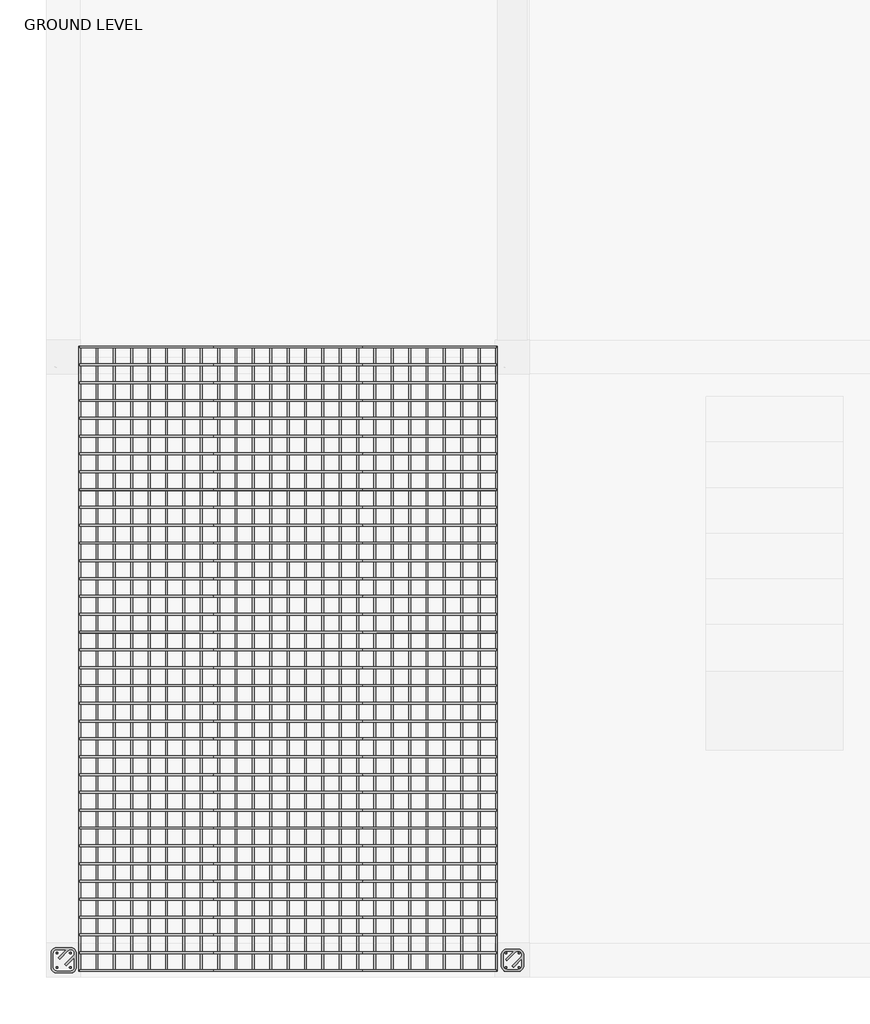
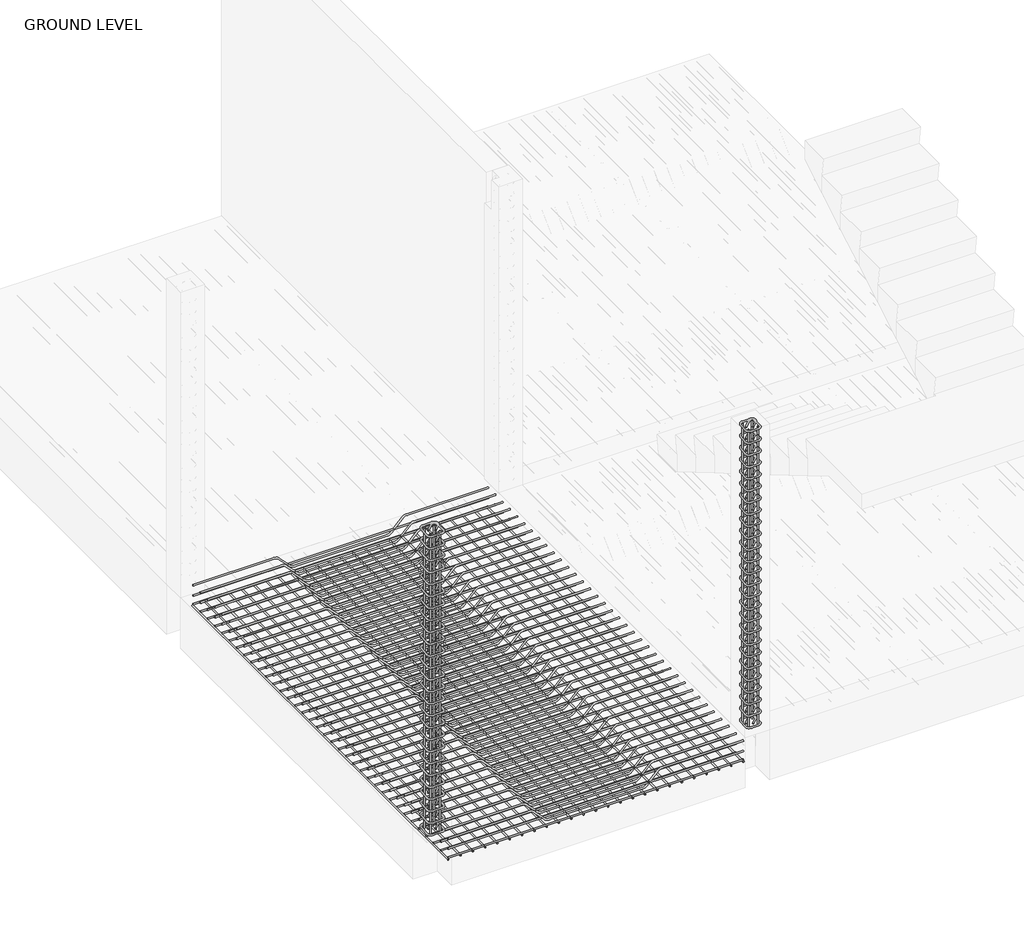
# One storey, part 2 of 8: 10 reinforcing bars.
"""IFC4 building model written with IfcOpenShell, lengths in millimetres."""

from ifc_helpers import new_model, si_unit, point, frame, origin, place, context, project, spatial, polyline, circle_curve, trimmed, segment, composite_curve, source, transform, mapped, element, save
from ifc_brep_helpers import swept_disk

model = new_model("IFC4")

# Units and contexts
model_context = context("Model", 3, world=origin())
ifc_project = project(units=[si_unit("LENGTHUNIT", "METRE", prefix="MILLI")], contexts=[model_context])

# Site, building, storey
site = spatial("IfcSite", under=ifc_project)
building = spatial("IfcBuilding", under=site)
storey = spatial("IfcBuildingStorey", under=building, Name="GROUND LEVEL", Elevation=0.0)

# Reinforcing bars
placement = place(None, origin())
reinforcing_bar_shape = source(origin(), model_context, "Body", "SolidModel", [
    swept_disk(composite_curve([segment(polyline([(-14816.7556793, -164.7525279, -60.0), (-14046.7544785, -164.7525279, -60.0)]), True, "CONTINUOUS"), segment(trimmed(circle_curve(frame((-14046.7544785, -164.7525279, -106.35), z_axis=(0.0, 1.0, 0.0), x_axis=(0.0, 0.0, 46.349999999999994)), 46.35), [point((-14046.7544785, -164.7525279, -60.0))], [point((-14013.9800792, -164.7525279, -73.5756007))], True, "CARTESIAN"), True, "CONTINUOUS"), segment(polyline([(-14013.9800792, -164.7525279, -73.5756007), (-13899.7099243, -164.7525279, -187.8457555)]), True, "CONTINUOUS"), segment(trimmed(circle_curve(frame((-13866.935525, -164.7525279, -155.0713562), z_axis=(0.0, -1.0, 0.0), x_axis=(-32.77439929999855, 0.0, -32.7743993)), 46.35), [point((-13899.7099243, -164.7525279, -187.8457555))], [point((-13866.935525, -164.7525279, -201.4213562))], True, "CARTESIAN"), True, "CONTINUOUS"), segment(polyline([(-13866.935525, -164.7525279, -201.4213562), (-12983.3758347, -164.7525279, -201.4213562)]), True, "CONTINUOUS"), segment(trimmed(circle_curve(frame((-12983.3758347, -164.7525279, -155.0713562), z_axis=(0.0, -1.0, 0.0), x_axis=(0.0, 0.0, -46.349999999999994)), 46.35), [point((-12983.3758347, -164.7525279, -201.4213562))], [point((-12950.6014354, -164.7525279, -187.8457555))], True, "CARTESIAN"), True, "CONTINUOUS"), segment(polyline([(-12950.6014354, -164.7525279, -187.8457555), (-12836.3312806, -164.7525279, -73.5756007)]), True, "CONTINUOUS"), segment(trimmed(circle_curve(frame((-12803.5568813, -164.7525279, -106.35), z_axis=(0.0, 1.0, 0.0), x_axis=(-32.77439929999855, 0.0, 32.7743993)), 46.35), [point((-12836.3312806, -164.7525279, -73.5756007))], [point((-12803.5568813, -164.7525279, -60.0))], True, "CARTESIAN"), True, "CONTINUOUS"), segment(polyline([(-12803.5568813, -164.7525279, -60.0), (-12033.5556805, -164.7525279, -60.0)]), True, "CONTINUOUS")], self_intersect=False), 6.35),
])
element("IfcReinforcingBar", 1, at=placement, inside=storey, context=model_context, shape_type="MappedRepresentation", body=[
    mapped(reinforcing_bar_shape, transform((0.0, 0.0, 0.0), x_axis=(1.0, 0.0, 0.0), y_axis=(0.0, 1.0, 0.0), z_axis=(0.0, 0.0, 1.0))),
    mapped(reinforcing_bar_shape, transform((0.0, -118.9455945, 0.0), x_axis=(1.0, 0.0, 0.0), y_axis=(0.0, 1.0, 0.0), z_axis=(0.0, 0.0, 1.0))),
    mapped(reinforcing_bar_shape, transform((0.0, -237.891189, 0.0), x_axis=(1.0, 0.0, 0.0), y_axis=(0.0, 1.0, 0.0), z_axis=(0.0, 0.0, 1.0))),
    mapped(reinforcing_bar_shape, transform((0.0, -356.8367835, 0.0), x_axis=(1.0, 0.0, 0.0), y_axis=(0.0, 1.0, 0.0), z_axis=(0.0, 0.0, 1.0))),
    mapped(reinforcing_bar_shape, transform((0.0, -475.7823779, 0.0), x_axis=(1.0, 0.0, 0.0), y_axis=(0.0, 1.0, 0.0), z_axis=(0.0, 0.0, 1.0))),
    mapped(reinforcing_bar_shape, transform((0.0, -594.7279724, 0.0), x_axis=(1.0, 0.0, 0.0), y_axis=(0.0, 1.0, 0.0), z_axis=(0.0, 0.0, 1.0))),
    mapped(reinforcing_bar_shape, transform((0.0, -713.6735669, 0.0), x_axis=(1.0, 0.0, 0.0), y_axis=(0.0, 1.0, 0.0), z_axis=(0.0, 0.0, 1.0))),
    mapped(reinforcing_bar_shape, transform((0.0, -832.6191614, 0.0), x_axis=(1.0, 0.0, 0.0), y_axis=(0.0, 1.0, 0.0), z_axis=(0.0, 0.0, 1.0))),
    mapped(reinforcing_bar_shape, transform((0.0, -951.5647559, 0.0), x_axis=(1.0, 0.0, 0.0), y_axis=(0.0, 1.0, 0.0), z_axis=(0.0, 0.0, 1.0))),
    mapped(reinforcing_bar_shape, transform((0.0, -1070.5103504, 0.0), x_axis=(1.0, 0.0, 0.0), y_axis=(0.0, 1.0, 0.0), z_axis=(0.0, 0.0, 1.0))),
    mapped(reinforcing_bar_shape, transform((0.0, -1189.4559449, 0.0), x_axis=(1.0, 0.0, 0.0), y_axis=(0.0, 1.0, 0.0), z_axis=(0.0, 0.0, 1.0))),
    mapped(reinforcing_bar_shape, transform((0.0, -1308.4015394, 0.0), x_axis=(1.0, 0.0, 0.0), y_axis=(0.0, 1.0, 0.0), z_axis=(0.0, 0.0, 1.0))),
    mapped(reinforcing_bar_shape, transform((0.0, -1427.3471338, 0.0), x_axis=(1.0, 0.0, 0.0), y_axis=(0.0, 1.0, 0.0), z_axis=(0.0, 0.0, 1.0))),
    mapped(reinforcing_bar_shape, transform((0.0, -1546.2927283, 0.0), x_axis=(1.0, 0.0, 0.0), y_axis=(0.0, 1.0, 0.0), z_axis=(0.0, 0.0, 1.0))),
    mapped(reinforcing_bar_shape, transform((0.0, -1665.2383228, 0.0), x_axis=(1.0, 0.0, 0.0), y_axis=(0.0, 1.0, 0.0), z_axis=(0.0, 0.0, 1.0))),
    mapped(reinforcing_bar_shape, transform((0.0, -1784.1839173, 0.0), x_axis=(1.0, 0.0, 0.0), y_axis=(0.0, 1.0, 0.0), z_axis=(0.0, 0.0, 1.0))),
    mapped(reinforcing_bar_shape, transform((0.0, -1903.1295118, 0.0), x_axis=(1.0, 0.0, 0.0), y_axis=(0.0, 1.0, 0.0), z_axis=(0.0, 0.0, 1.0))),
    mapped(reinforcing_bar_shape, transform((0.0, -2022.0751063, 0.0), x_axis=(1.0, 0.0, 0.0), y_axis=(0.0, 1.0, 0.0), z_axis=(0.0, 0.0, 1.0))),
    mapped(reinforcing_bar_shape, transform((0.0, -2141.0207008, 0.0), x_axis=(1.0, 0.0, 0.0), y_axis=(0.0, 1.0, 0.0), z_axis=(0.0, 0.0, 1.0))),
    mapped(reinforcing_bar_shape, transform((0.0, -2259.9662953, 0.0), x_axis=(1.0, 0.0, 0.0), y_axis=(0.0, 1.0, 0.0), z_axis=(0.0, 0.0, 1.0))),
    mapped(reinforcing_bar_shape, transform((0.0, -2378.9118897, 0.0), x_axis=(1.0, 0.0, 0.0), y_axis=(0.0, 1.0, 0.0), z_axis=(0.0, 0.0, 1.0))),
    mapped(reinforcing_bar_shape, transform((0.0, -2497.8574842, 0.0), x_axis=(1.0, 0.0, 0.0), y_axis=(0.0, 1.0, 0.0), z_axis=(0.0, 0.0, 1.0))),
    mapped(reinforcing_bar_shape, transform((0.0, -2616.8030787, 0.0), x_axis=(1.0, 0.0, 0.0), y_axis=(0.0, 1.0, 0.0), z_axis=(0.0, 0.0, 1.0))),
    mapped(reinforcing_bar_shape, transform((0.0, -2735.7486732, 0.0), x_axis=(1.0, 0.0, 0.0), y_axis=(0.0, 1.0, 0.0), z_axis=(0.0, 0.0, 1.0))),
    mapped(reinforcing_bar_shape, transform((0.0, -2854.6942677, 0.0), x_axis=(1.0, 0.0, 0.0), y_axis=(0.0, 1.0, 0.0), z_axis=(0.0, 0.0, 1.0))),
    mapped(reinforcing_bar_shape, transform((0.0, -2973.6398622, 0.0), x_axis=(1.0, 0.0, 0.0), y_axis=(0.0, 1.0, 0.0), z_axis=(0.0, 0.0, 1.0))),
    mapped(reinforcing_bar_shape, transform((0.0, -3092.5854567, 0.0), x_axis=(1.0, 0.0, 0.0), y_axis=(0.0, 1.0, 0.0), z_axis=(0.0, 0.0, 1.0))),
    mapped(reinforcing_bar_shape, transform((0.0, -3211.5310511, 0.0), x_axis=(1.0, 0.0, 0.0), y_axis=(0.0, 1.0, 0.0), z_axis=(0.0, 0.0, 1.0))),
    mapped(reinforcing_bar_shape, transform((0.0, -3330.4766456, 0.0), x_axis=(1.0, 0.0, 0.0), y_axis=(0.0, 1.0, 0.0), z_axis=(0.0, 0.0, 1.0))),
    mapped(reinforcing_bar_shape, transform((0.0, -3449.4222401, 0.0), x_axis=(1.0, 0.0, 0.0), y_axis=(0.0, 1.0, 0.0), z_axis=(0.0, 0.0, 1.0))),
    mapped(reinforcing_bar_shape, transform((0.0, -3568.3678346, 0.0), x_axis=(1.0, 0.0, 0.0), y_axis=(0.0, 1.0, 0.0), z_axis=(0.0, 0.0, 1.0))),
    mapped(reinforcing_bar_shape, transform((0.0, -3687.3134291, 0.0), x_axis=(1.0, 0.0, 0.0), y_axis=(0.0, 1.0, 0.0), z_axis=(0.0, 0.0, 1.0))),
    mapped(reinforcing_bar_shape, transform((0.0, -3806.2590236, 0.0), x_axis=(1.0, 0.0, 0.0), y_axis=(0.0, 1.0, 0.0), z_axis=(0.0, 0.0, 1.0))),
    mapped(reinforcing_bar_shape, transform((0.0, -3925.2046181, 0.0), x_axis=(1.0, 0.0, 0.0), y_axis=(0.0, 1.0, 0.0), z_axis=(0.0, 0.0, 1.0))),
    mapped(reinforcing_bar_shape, transform((0.0, -4044.1502126, 0.0), x_axis=(1.0, 0.0, 0.0), y_axis=(0.0, 1.0, 0.0), z_axis=(0.0, 0.0, 1.0))),
    mapped(reinforcing_bar_shape, transform((0.0, -4163.095807, 0.0), x_axis=(1.0, 0.0, 0.0), y_axis=(0.0, 1.0, 0.0), z_axis=(0.0, 0.0, 1.0))),
])
reinforcing_bar_2_shape = source(origin(), model_context, "Body", "SolidModel", [
    swept_disk(composite_curve([segment(polyline([(-12033.5556805, -164.7525279, -249.9712592), (-14816.7556793, -164.7525279, -249.9712592)]), True, "CONTINUOUS")], self_intersect=False), 6.35),
])
element("IfcReinforcingBar", 2, at=placement, inside=storey, context=model_context, shape_type="MappedRepresentation", body=[
    mapped(reinforcing_bar_2_shape, transform((0.0, 0.0, 0.0), x_axis=(1.0, 0.0, 0.0), y_axis=(0.0, 1.0, 0.0), z_axis=(0.0, 0.0, 1.0))),
    mapped(reinforcing_bar_2_shape, transform((0.0, -118.9455945, 0.0), x_axis=(1.0, 0.0, 0.0), y_axis=(0.0, 1.0, 0.0), z_axis=(0.0, 0.0, 1.0))),
    mapped(reinforcing_bar_2_shape, transform((0.0, -237.891189, 0.0), x_axis=(1.0, 0.0, 0.0), y_axis=(0.0, 1.0, 0.0), z_axis=(0.0, 0.0, 1.0))),
    mapped(reinforcing_bar_2_shape, transform((0.0, -356.8367835, 0.0), x_axis=(1.0, 0.0, 0.0), y_axis=(0.0, 1.0, 0.0), z_axis=(0.0, 0.0, 1.0))),
    mapped(reinforcing_bar_2_shape, transform((0.0, -475.7823779, 0.0), x_axis=(1.0, 0.0, 0.0), y_axis=(0.0, 1.0, 0.0), z_axis=(0.0, 0.0, 1.0))),
    mapped(reinforcing_bar_2_shape, transform((0.0, -594.7279724, 0.0), x_axis=(1.0, 0.0, 0.0), y_axis=(0.0, 1.0, 0.0), z_axis=(0.0, 0.0, 1.0))),
    mapped(reinforcing_bar_2_shape, transform((0.0, -713.6735669, 0.0), x_axis=(1.0, 0.0, 0.0), y_axis=(0.0, 1.0, 0.0), z_axis=(0.0, 0.0, 1.0))),
    mapped(reinforcing_bar_2_shape, transform((0.0, -832.6191614, 0.0), x_axis=(1.0, 0.0, 0.0), y_axis=(0.0, 1.0, 0.0), z_axis=(0.0, 0.0, 1.0))),
    mapped(reinforcing_bar_2_shape, transform((0.0, -951.5647559, 0.0), x_axis=(1.0, 0.0, 0.0), y_axis=(0.0, 1.0, 0.0), z_axis=(0.0, 0.0, 1.0))),
    mapped(reinforcing_bar_2_shape, transform((0.0, -1070.5103504, 0.0), x_axis=(1.0, 0.0, 0.0), y_axis=(0.0, 1.0, 0.0), z_axis=(0.0, 0.0, 1.0))),
    mapped(reinforcing_bar_2_shape, transform((0.0, -1189.4559449, 0.0), x_axis=(1.0, 0.0, 0.0), y_axis=(0.0, 1.0, 0.0), z_axis=(0.0, 0.0, 1.0))),
    mapped(reinforcing_bar_2_shape, transform((0.0, -1308.4015394, 0.0), x_axis=(1.0, 0.0, 0.0), y_axis=(0.0, 1.0, 0.0), z_axis=(0.0, 0.0, 1.0))),
    mapped(reinforcing_bar_2_shape, transform((0.0, -1427.3471338, 0.0), x_axis=(1.0, 0.0, 0.0), y_axis=(0.0, 1.0, 0.0), z_axis=(0.0, 0.0, 1.0))),
    mapped(reinforcing_bar_2_shape, transform((0.0, -1546.2927283, 0.0), x_axis=(1.0, 0.0, 0.0), y_axis=(0.0, 1.0, 0.0), z_axis=(0.0, 0.0, 1.0))),
    mapped(reinforcing_bar_2_shape, transform((0.0, -1665.2383228, 0.0), x_axis=(1.0, 0.0, 0.0), y_axis=(0.0, 1.0, 0.0), z_axis=(0.0, 0.0, 1.0))),
    mapped(reinforcing_bar_2_shape, transform((0.0, -1784.1839173, 0.0), x_axis=(1.0, 0.0, 0.0), y_axis=(0.0, 1.0, 0.0), z_axis=(0.0, 0.0, 1.0))),
    mapped(reinforcing_bar_2_shape, transform((0.0, -1903.1295118, 0.0), x_axis=(1.0, 0.0, 0.0), y_axis=(0.0, 1.0, 0.0), z_axis=(0.0, 0.0, 1.0))),
    mapped(reinforcing_bar_2_shape, transform((0.0, -2022.0751063, 0.0), x_axis=(1.0, 0.0, 0.0), y_axis=(0.0, 1.0, 0.0), z_axis=(0.0, 0.0, 1.0))),
    mapped(reinforcing_bar_2_shape, transform((0.0, -2141.0207008, 0.0), x_axis=(1.0, 0.0, 0.0), y_axis=(0.0, 1.0, 0.0), z_axis=(0.0, 0.0, 1.0))),
    mapped(reinforcing_bar_2_shape, transform((0.0, -2259.9662953, 0.0), x_axis=(1.0, 0.0, 0.0), y_axis=(0.0, 1.0, 0.0), z_axis=(0.0, 0.0, 1.0))),
    mapped(reinforcing_bar_2_shape, transform((0.0, -2378.9118897, 0.0), x_axis=(1.0, 0.0, 0.0), y_axis=(0.0, 1.0, 0.0), z_axis=(0.0, 0.0, 1.0))),
    mapped(reinforcing_bar_2_shape, transform((0.0, -2497.8574842, 0.0), x_axis=(1.0, 0.0, 0.0), y_axis=(0.0, 1.0, 0.0), z_axis=(0.0, 0.0, 1.0))),
    mapped(reinforcing_bar_2_shape, transform((0.0, -2616.8030787, 0.0), x_axis=(1.0, 0.0, 0.0), y_axis=(0.0, 1.0, 0.0), z_axis=(0.0, 0.0, 1.0))),
    mapped(reinforcing_bar_2_shape, transform((0.0, -2735.7486732, 0.0), x_axis=(1.0, 0.0, 0.0), y_axis=(0.0, 1.0, 0.0), z_axis=(0.0, 0.0, 1.0))),
    mapped(reinforcing_bar_2_shape, transform((0.0, -2854.6942677, 0.0), x_axis=(1.0, 0.0, 0.0), y_axis=(0.0, 1.0, 0.0), z_axis=(0.0, 0.0, 1.0))),
    mapped(reinforcing_bar_2_shape, transform((0.0, -2973.6398622, 0.0), x_axis=(1.0, 0.0, 0.0), y_axis=(0.0, 1.0, 0.0), z_axis=(0.0, 0.0, 1.0))),
    mapped(reinforcing_bar_2_shape, transform((0.0, -3092.5854567, 0.0), x_axis=(1.0, 0.0, 0.0), y_axis=(0.0, 1.0, 0.0), z_axis=(0.0, 0.0, 1.0))),
    mapped(reinforcing_bar_2_shape, transform((0.0, -3211.5310511, 0.0), x_axis=(1.0, 0.0, 0.0), y_axis=(0.0, 1.0, 0.0), z_axis=(0.0, 0.0, 1.0))),
    mapped(reinforcing_bar_2_shape, transform((0.0, -3330.4766456, 0.0), x_axis=(1.0, 0.0, 0.0), y_axis=(0.0, 1.0, 0.0), z_axis=(0.0, 0.0, 1.0))),
    mapped(reinforcing_bar_2_shape, transform((0.0, -3449.4222401, 0.0), x_axis=(1.0, 0.0, 0.0), y_axis=(0.0, 1.0, 0.0), z_axis=(0.0, 0.0, 1.0))),
    mapped(reinforcing_bar_2_shape, transform((0.0, -3568.3678346, 0.0), x_axis=(1.0, 0.0, 0.0), y_axis=(0.0, 1.0, 0.0), z_axis=(0.0, 0.0, 1.0))),
    mapped(reinforcing_bar_2_shape, transform((0.0, -3687.3134291, 0.0), x_axis=(1.0, 0.0, 0.0), y_axis=(0.0, 1.0, 0.0), z_axis=(0.0, 0.0, 1.0))),
    mapped(reinforcing_bar_2_shape, transform((0.0, -3806.2590236, 0.0), x_axis=(1.0, 0.0, 0.0), y_axis=(0.0, 1.0, 0.0), z_axis=(0.0, 0.0, 1.0))),
    mapped(reinforcing_bar_2_shape, transform((0.0, -3925.2046181, 0.0), x_axis=(1.0, 0.0, 0.0), y_axis=(0.0, 1.0, 0.0), z_axis=(0.0, 0.0, 1.0))),
    mapped(reinforcing_bar_2_shape, transform((0.0, -4044.1502126, 0.0), x_axis=(1.0, 0.0, 0.0), y_axis=(0.0, 1.0, 0.0), z_axis=(0.0, 0.0, 1.0))),
    mapped(reinforcing_bar_2_shape, transform((0.0, -4163.095807, 0.0), x_axis=(1.0, 0.0, 0.0), y_axis=(0.0, 1.0, 0.0), z_axis=(0.0, 0.0, 1.0))),
])
reinforcing_bar_3_shape = source(origin(), model_context, "Body", "SolidModel", [
    swept_disk(composite_curve([segment(polyline([(-14816.7556793, -164.7525279, -161.5623157), (-12033.5556805, -164.7525279, -161.5623157)]), True, "CONTINUOUS")], self_intersect=False), 6.35),
])
element("IfcReinforcingBar", 3, at=placement, inside=storey, context=model_context, shape_type="MappedRepresentation", body=[
    mapped(reinforcing_bar_3_shape, transform((0.0, 0.0, 0.0), x_axis=(1.0, 0.0, 0.0), y_axis=(0.0, 1.0, 0.0), z_axis=(0.0, 0.0, 1.0))),
    mapped(reinforcing_bar_3_shape, transform((0.0, -118.9455945, 0.0), x_axis=(1.0, 0.0, 0.0), y_axis=(0.0, 1.0, 0.0), z_axis=(0.0, 0.0, 1.0))),
    mapped(reinforcing_bar_3_shape, transform((0.0, -237.891189, 0.0), x_axis=(1.0, 0.0, 0.0), y_axis=(0.0, 1.0, 0.0), z_axis=(0.0, 0.0, 1.0))),
    mapped(reinforcing_bar_3_shape, transform((0.0, -356.8367835, 0.0), x_axis=(1.0, 0.0, 0.0), y_axis=(0.0, 1.0, 0.0), z_axis=(0.0, 0.0, 1.0))),
    mapped(reinforcing_bar_3_shape, transform((0.0, -475.7823779, 0.0), x_axis=(1.0, 0.0, 0.0), y_axis=(0.0, 1.0, 0.0), z_axis=(0.0, 0.0, 1.0))),
    mapped(reinforcing_bar_3_shape, transform((0.0, -594.7279724, 0.0), x_axis=(1.0, 0.0, 0.0), y_axis=(0.0, 1.0, 0.0), z_axis=(0.0, 0.0, 1.0))),
    mapped(reinforcing_bar_3_shape, transform((0.0, -713.6735669, 0.0), x_axis=(1.0, 0.0, 0.0), y_axis=(0.0, 1.0, 0.0), z_axis=(0.0, 0.0, 1.0))),
    mapped(reinforcing_bar_3_shape, transform((0.0, -832.6191614, 0.0), x_axis=(1.0, 0.0, 0.0), y_axis=(0.0, 1.0, 0.0), z_axis=(0.0, 0.0, 1.0))),
    mapped(reinforcing_bar_3_shape, transform((0.0, -951.5647559, 0.0), x_axis=(1.0, 0.0, 0.0), y_axis=(0.0, 1.0, 0.0), z_axis=(0.0, 0.0, 1.0))),
    mapped(reinforcing_bar_3_shape, transform((0.0, -1070.5103504, 0.0), x_axis=(1.0, 0.0, 0.0), y_axis=(0.0, 1.0, 0.0), z_axis=(0.0, 0.0, 1.0))),
    mapped(reinforcing_bar_3_shape, transform((0.0, -1189.4559449, 0.0), x_axis=(1.0, 0.0, 0.0), y_axis=(0.0, 1.0, 0.0), z_axis=(0.0, 0.0, 1.0))),
    mapped(reinforcing_bar_3_shape, transform((0.0, -1308.4015394, 0.0), x_axis=(1.0, 0.0, 0.0), y_axis=(0.0, 1.0, 0.0), z_axis=(0.0, 0.0, 1.0))),
    mapped(reinforcing_bar_3_shape, transform((0.0, -1427.3471338, 0.0), x_axis=(1.0, 0.0, 0.0), y_axis=(0.0, 1.0, 0.0), z_axis=(0.0, 0.0, 1.0))),
    mapped(reinforcing_bar_3_shape, transform((0.0, -1546.2927283, 0.0), x_axis=(1.0, 0.0, 0.0), y_axis=(0.0, 1.0, 0.0), z_axis=(0.0, 0.0, 1.0))),
    mapped(reinforcing_bar_3_shape, transform((0.0, -1665.2383228, 0.0), x_axis=(1.0, 0.0, 0.0), y_axis=(0.0, 1.0, 0.0), z_axis=(0.0, 0.0, 1.0))),
    mapped(reinforcing_bar_3_shape, transform((0.0, -1784.1839173, 0.0), x_axis=(1.0, 0.0, 0.0), y_axis=(0.0, 1.0, 0.0), z_axis=(0.0, 0.0, 1.0))),
    mapped(reinforcing_bar_3_shape, transform((0.0, -1903.1295118, 0.0), x_axis=(1.0, 0.0, 0.0), y_axis=(0.0, 1.0, 0.0), z_axis=(0.0, 0.0, 1.0))),
    mapped(reinforcing_bar_3_shape, transform((0.0, -2022.0751063, 0.0), x_axis=(1.0, 0.0, 0.0), y_axis=(0.0, 1.0, 0.0), z_axis=(0.0, 0.0, 1.0))),
    mapped(reinforcing_bar_3_shape, transform((0.0, -2141.0207008, 0.0), x_axis=(1.0, 0.0, 0.0), y_axis=(0.0, 1.0, 0.0), z_axis=(0.0, 0.0, 1.0))),
    mapped(reinforcing_bar_3_shape, transform((0.0, -2259.9662953, 0.0), x_axis=(1.0, 0.0, 0.0), y_axis=(0.0, 1.0, 0.0), z_axis=(0.0, 0.0, 1.0))),
    mapped(reinforcing_bar_3_shape, transform((0.0, -2378.9118897, 0.0), x_axis=(1.0, 0.0, 0.0), y_axis=(0.0, 1.0, 0.0), z_axis=(0.0, 0.0, 1.0))),
    mapped(reinforcing_bar_3_shape, transform((0.0, -2497.8574842, 0.0), x_axis=(1.0, 0.0, 0.0), y_axis=(0.0, 1.0, 0.0), z_axis=(0.0, 0.0, 1.0))),
    mapped(reinforcing_bar_3_shape, transform((0.0, -2616.8030787, 0.0), x_axis=(1.0, 0.0, 0.0), y_axis=(0.0, 1.0, 0.0), z_axis=(0.0, 0.0, 1.0))),
    mapped(reinforcing_bar_3_shape, transform((0.0, -2735.7486732, 0.0), x_axis=(1.0, 0.0, 0.0), y_axis=(0.0, 1.0, 0.0), z_axis=(0.0, 0.0, 1.0))),
    mapped(reinforcing_bar_3_shape, transform((0.0, -2854.6942677, 0.0), x_axis=(1.0, 0.0, 0.0), y_axis=(0.0, 1.0, 0.0), z_axis=(0.0, 0.0, 1.0))),
    mapped(reinforcing_bar_3_shape, transform((0.0, -2973.6398622, 0.0), x_axis=(1.0, 0.0, 0.0), y_axis=(0.0, 1.0, 0.0), z_axis=(0.0, 0.0, 1.0))),
    mapped(reinforcing_bar_3_shape, transform((0.0, -3092.5854567, 0.0), x_axis=(1.0, 0.0, 0.0), y_axis=(0.0, 1.0, 0.0), z_axis=(0.0, 0.0, 1.0))),
    mapped(reinforcing_bar_3_shape, transform((0.0, -3211.5310511, 0.0), x_axis=(1.0, 0.0, 0.0), y_axis=(0.0, 1.0, 0.0), z_axis=(0.0, 0.0, 1.0))),
    mapped(reinforcing_bar_3_shape, transform((0.0, -3330.4766456, 0.0), x_axis=(1.0, 0.0, 0.0), y_axis=(0.0, 1.0, 0.0), z_axis=(0.0, 0.0, 1.0))),
    mapped(reinforcing_bar_3_shape, transform((0.0, -3449.4222401, 0.0), x_axis=(1.0, 0.0, 0.0), y_axis=(0.0, 1.0, 0.0), z_axis=(0.0, 0.0, 1.0))),
    mapped(reinforcing_bar_3_shape, transform((0.0, -3568.3678346, 0.0), x_axis=(1.0, 0.0, 0.0), y_axis=(0.0, 1.0, 0.0), z_axis=(0.0, 0.0, 1.0))),
    mapped(reinforcing_bar_3_shape, transform((0.0, -3687.3134291, 0.0), x_axis=(1.0, 0.0, 0.0), y_axis=(0.0, 1.0, 0.0), z_axis=(0.0, 0.0, 1.0))),
    mapped(reinforcing_bar_3_shape, transform((0.0, -3806.2590236, 0.0), x_axis=(1.0, 0.0, 0.0), y_axis=(0.0, 1.0, 0.0), z_axis=(0.0, 0.0, 1.0))),
    mapped(reinforcing_bar_3_shape, transform((0.0, -3925.2046181, 0.0), x_axis=(1.0, 0.0, 0.0), y_axis=(0.0, 1.0, 0.0), z_axis=(0.0, 0.0, 1.0))),
    mapped(reinforcing_bar_3_shape, transform((0.0, -4044.1502126, 0.0), x_axis=(1.0, 0.0, 0.0), y_axis=(0.0, 1.0, 0.0), z_axis=(0.0, 0.0, 1.0))),
    mapped(reinforcing_bar_3_shape, transform((0.0, -4163.095807, 0.0), x_axis=(1.0, 0.0, 0.0), y_axis=(0.0, 1.0, 0.0), z_axis=(0.0, 0.0, 1.0))),
])
reinforcing_bar_4_shape = source(origin(), model_context, "Body", "SolidModel", [
    swept_disk(composite_curve([segment(polyline([(-14816.7556793, -158.4025279, -265.2544844), (-14816.7556793, -4334.1983349, -265.2544844)]), True, "CONTINUOUS")], self_intersect=False), 6.35),
])
element("IfcReinforcingBar", 4, at=placement, inside=storey, context=model_context, shape_type="MappedRepresentation", body=[
    mapped(reinforcing_bar_4_shape, transform((0.0, 0.0, 0.0), x_axis=(1.0, 0.0, 0.0), y_axis=(0.0, 1.0, 0.0), z_axis=(0.0, 0.0, 1.0))),
    mapped(reinforcing_bar_4_shape, transform((115.9666666, 0.0, 0.0), x_axis=(1.0, 0.0, 0.0), y_axis=(0.0, 1.0, 0.0), z_axis=(0.0, 0.0, 1.0))),
    mapped(reinforcing_bar_4_shape, transform((231.9333332, 0.0, 0.0), x_axis=(1.0, 0.0, 0.0), y_axis=(0.0, 1.0, 0.0), z_axis=(0.0, 0.0, 1.0))),
    mapped(reinforcing_bar_4_shape, transform((347.8999998, 0.0, 0.0), x_axis=(1.0, 0.0, 0.0), y_axis=(0.0, 1.0, 0.0), z_axis=(0.0, 0.0, 1.0))),
    mapped(reinforcing_bar_4_shape, transform((463.8666665, 0.0, 0.0), x_axis=(1.0, 0.0, 0.0), y_axis=(0.0, 1.0, 0.0), z_axis=(0.0, 0.0, 1.0))),
    mapped(reinforcing_bar_4_shape, transform((579.8333331, 0.0, 0.0), x_axis=(1.0, 0.0, 0.0), y_axis=(0.0, 1.0, 0.0), z_axis=(0.0, 0.0, 1.0))),
    mapped(reinforcing_bar_4_shape, transform((695.7999997, 0.0, 0.0), x_axis=(1.0, 0.0, 0.0), y_axis=(0.0, 1.0, 0.0), z_axis=(0.0, 0.0, 1.0))),
    mapped(reinforcing_bar_4_shape, transform((811.7666663, 0.0, 0.0), x_axis=(1.0, 0.0, 0.0), y_axis=(0.0, 1.0, 0.0), z_axis=(0.0, 0.0, 1.0))),
    mapped(reinforcing_bar_4_shape, transform((927.7333329, 0.0, 0.0), x_axis=(1.0, 0.0, 0.0), y_axis=(0.0, 1.0, 0.0), z_axis=(0.0, 0.0, 1.0))),
    mapped(reinforcing_bar_4_shape, transform((1043.6999995, 0.0, 0.0), x_axis=(1.0, 0.0, 0.0), y_axis=(0.0, 1.0, 0.0), z_axis=(0.0, 0.0, 1.0))),
    mapped(reinforcing_bar_4_shape, transform((1159.6666662, 0.0, 0.0), x_axis=(1.0, 0.0, 0.0), y_axis=(0.0, 1.0, 0.0), z_axis=(0.0, 0.0, 1.0))),
    mapped(reinforcing_bar_4_shape, transform((1275.6333328, 0.0, 0.0), x_axis=(1.0, 0.0, 0.0), y_axis=(0.0, 1.0, 0.0), z_axis=(0.0, 0.0, 1.0))),
    mapped(reinforcing_bar_4_shape, transform((1391.5999994, 0.0, 0.0), x_axis=(1.0, 0.0, 0.0), y_axis=(0.0, 1.0, 0.0), z_axis=(0.0, 0.0, 1.0))),
    mapped(reinforcing_bar_4_shape, transform((1507.566666, 0.0, 0.0), x_axis=(1.0, 0.0, 0.0), y_axis=(0.0, 1.0, 0.0), z_axis=(0.0, 0.0, 1.0))),
    mapped(reinforcing_bar_4_shape, transform((1623.5333326, 0.0, 0.0), x_axis=(1.0, 0.0, 0.0), y_axis=(0.0, 1.0, 0.0), z_axis=(0.0, 0.0, 1.0))),
    mapped(reinforcing_bar_4_shape, transform((1739.4999992, 0.0, 0.0), x_axis=(1.0, 0.0, 0.0), y_axis=(0.0, 1.0, 0.0), z_axis=(0.0, 0.0, 1.0))),
    mapped(reinforcing_bar_4_shape, transform((1855.4666659, 0.0, 0.0), x_axis=(1.0, 0.0, 0.0), y_axis=(0.0, 1.0, 0.0), z_axis=(0.0, 0.0, 1.0))),
    mapped(reinforcing_bar_4_shape, transform((1971.4333325, 0.0, 0.0), x_axis=(1.0, 0.0, 0.0), y_axis=(0.0, 1.0, 0.0), z_axis=(0.0, 0.0, 1.0))),
    mapped(reinforcing_bar_4_shape, transform((2087.3999991, 0.0, 0.0), x_axis=(1.0, 0.0, 0.0), y_axis=(0.0, 1.0, 0.0), z_axis=(0.0, 0.0, 1.0))),
    mapped(reinforcing_bar_4_shape, transform((2203.3666657, 0.0, 0.0), x_axis=(1.0, 0.0, 0.0), y_axis=(0.0, 1.0, 0.0), z_axis=(0.0, 0.0, 1.0))),
    mapped(reinforcing_bar_4_shape, transform((2319.3333323, 0.0, 0.0), x_axis=(1.0, 0.0, 0.0), y_axis=(0.0, 1.0, 0.0), z_axis=(0.0, 0.0, 1.0))),
    mapped(reinforcing_bar_4_shape, transform((2435.2999989, 0.0, 0.0), x_axis=(1.0, 0.0, 0.0), y_axis=(0.0, 1.0, 0.0), z_axis=(0.0, 0.0, 1.0))),
    mapped(reinforcing_bar_4_shape, transform((2551.2666655, 0.0, 0.0), x_axis=(1.0, 0.0, 0.0), y_axis=(0.0, 1.0, 0.0), z_axis=(0.0, 0.0, 1.0))),
    mapped(reinforcing_bar_4_shape, transform((2667.2333322, 0.0, 0.0), x_axis=(1.0, 0.0, 0.0), y_axis=(0.0, 1.0, 0.0), z_axis=(0.0, 0.0, 1.0))),
    mapped(reinforcing_bar_4_shape, transform((2783.1999988, 0.0, 0.0), x_axis=(1.0, 0.0, 0.0), y_axis=(0.0, 1.0, 0.0), z_axis=(0.0, 0.0, 1.0))),
])
reinforcing_bar_5_shape = source(origin(), model_context, "Body", "SolidModel", [
    swept_disk(composite_curve([segment(polyline([(-11881.8006936, -4211.1006392, 3008.0), (-11881.8006936, -4211.1006392, 40.0)]), True, "CONTINUOUS")], self_intersect=False), 6.35),
])
element("IfcReinforcingBar", 5, at=placement, inside=storey, context=model_context, shape_type="MappedRepresentation", body=[
    mapped(reinforcing_bar_5_shape, transform((0.0, 0.0, 0.0), x_axis=(1.0, 0.0, 0.0), y_axis=(0.0, 1.0, 0.0), z_axis=(0.0, 0.0, 1.0))),
    mapped(reinforcing_bar_5_shape, transform((0.0, -96.9916148, 0.0), x_axis=(1.0, 0.0, 0.0), y_axis=(0.0, 1.0, 0.0), z_axis=(0.0, 0.0, 1.0))),
])
reinforcing_bar_6_shape = source(origin(), model_context, "Body", "SolidModel", [
    swept_disk(composite_curve([segment(polyline([(-11967.8670404, -4256.8741003, 3001.65), (-11912.1234775, -4201.1305373, 3001.65)]), True, "CONTINUOUS"), segment(trimmed(circle_curve(frame((-11889.9556799, -4223.2983349, 3001.65), z_axis=(0.0, 0.0, -1.0), x_axis=(-22.167797599999176, 22.167797600000085, 0.0)), 31.35), [point((-11912.1234775, -4201.1305373, 3001.65))], [point((-11858.6056799, -4223.2983349, 3001.65))], True, "CARTESIAN"), True, "CONTINUOUS"), segment(polyline([(-11858.6056799, -4223.2983349, 3001.65), (-11858.6056799, -4296.4983349, 3001.65)]), True, "CONTINUOUS"), segment(trimmed(circle_curve(frame((-11889.9556799, -4296.4983349, 3001.65), z_axis=(0.0, 0.0, -1.0), x_axis=(31.350000000000364, 0.0, 0.0)), 31.35), [point((-11858.6056799, -4296.4983349, 3001.65))], [point((-11889.9556799, -4327.8483349, 3001.65))], True, "CARTESIAN"), True, "CONTINUOUS"), segment(polyline([(-11889.9556799, -4327.8483349, 3001.65), (-11963.1556799, -4327.8483349, 3001.65)]), True, "CONTINUOUS"), segment(trimmed(circle_curve(frame((-11963.1556799, -4296.6343361, 3004.5669815), z_axis=(0.0, 0.09304566152621355, -0.9956618426308951), x_axis=(0.0, -31.2139987999999, -2.91698150000002)), 31.35), [point((-11963.1556799, -4327.8483349, 3001.65))], [point((-11994.5056799, -4296.6343361, 3004.5669815))], True, "CARTESIAN"), True, "CONTINUOUS"), segment(polyline([(-11994.5056799, -4296.6343361, 3004.5669815), (-11994.5056799, -4223.1623337, 3011.4330185)]), True, "CONTINUOUS"), segment(trimmed(circle_curve(frame((-11963.1556799, -4223.1623337, 3011.4330185), z_axis=(0.0, 0.09304566152621355, -0.9956618426308951), x_axis=(-31.349999999998545, 0.0, 0.0)), 31.35), [point((-11994.5056799, -4223.1623337, 3011.4330185))], [point((-11963.1556799, -4191.9483349, 3014.35))], True, "CARTESIAN"), True, "CONTINUOUS"), segment(polyline([(-11963.1556799, -4191.9483349, 3014.35), (-11889.9556799, -4191.9483349, 3014.35)]), True, "CONTINUOUS"), segment(trimmed(circle_curve(frame((-11889.9556799, -4223.2983349, 3014.35), z_axis=(0.0, 0.0, -1.0), x_axis=(0.0, 31.349999999999454, 0.0)), 31.35), [point((-11889.9556799, -4191.9483349, 3014.35))], [point((-11867.7878823, -4245.4661325, 3014.35))], True, "CARTESIAN"), True, "CONTINUOUS"), segment(polyline([(-11867.7878823, -4245.4661325, 3014.35), (-11923.5314452, -4301.2096954, 3014.35)]), True, "CONTINUOUS")], self_intersect=False), 6.35),
])
element("IfcReinforcingBar", 6, at=placement, inside=storey, context=model_context, shape_type="MappedRepresentation", body=[
    mapped(reinforcing_bar_6_shape, transform((0.0, 0.0, 0.0), x_axis=(1.0, 0.0, 0.0), y_axis=(0.0, 1.0, 0.0), z_axis=(0.0, 0.0, 1.0))),
    mapped(reinforcing_bar_6_shape, transform((0.0, 0.0, -118.212), x_axis=(1.0, 0.0, 0.0), y_axis=(0.0, 1.0, 0.0), z_axis=(0.0, 0.0, 1.0))),
    mapped(reinforcing_bar_6_shape, transform((0.0, 0.0, -236.424), x_axis=(1.0, 0.0, 0.0), y_axis=(0.0, 1.0, 0.0), z_axis=(0.0, 0.0, 1.0))),
    mapped(reinforcing_bar_6_shape, transform((0.0, 0.0, -354.636), x_axis=(1.0, 0.0, 0.0), y_axis=(0.0, 1.0, 0.0), z_axis=(0.0, 0.0, 1.0))),
    mapped(reinforcing_bar_6_shape, transform((0.0, 0.0, -472.848), x_axis=(1.0, 0.0, 0.0), y_axis=(0.0, 1.0, 0.0), z_axis=(0.0, 0.0, 1.0))),
    mapped(reinforcing_bar_6_shape, transform((0.0, 0.0, -591.06), x_axis=(1.0, 0.0, 0.0), y_axis=(0.0, 1.0, 0.0), z_axis=(0.0, 0.0, 1.0))),
    mapped(reinforcing_bar_6_shape, transform((0.0, 0.0, -709.272), x_axis=(1.0, 0.0, 0.0), y_axis=(0.0, 1.0, 0.0), z_axis=(0.0, 0.0, 1.0))),
    mapped(reinforcing_bar_6_shape, transform((0.0, 0.0, -827.484), x_axis=(1.0, 0.0, 0.0), y_axis=(0.0, 1.0, 0.0), z_axis=(0.0, 0.0, 1.0))),
    mapped(reinforcing_bar_6_shape, transform((0.0, 0.0, -945.696), x_axis=(1.0, 0.0, 0.0), y_axis=(0.0, 1.0, 0.0), z_axis=(0.0, 0.0, 1.0))),
    mapped(reinforcing_bar_6_shape, transform((0.0, 0.0, -1063.908), x_axis=(1.0, 0.0, 0.0), y_axis=(0.0, 1.0, 0.0), z_axis=(0.0, 0.0, 1.0))),
    mapped(reinforcing_bar_6_shape, transform((0.0, 0.0, -1182.12), x_axis=(1.0, 0.0, 0.0), y_axis=(0.0, 1.0, 0.0), z_axis=(0.0, 0.0, 1.0))),
    mapped(reinforcing_bar_6_shape, transform((0.0, 0.0, -1300.332), x_axis=(1.0, 0.0, 0.0), y_axis=(0.0, 1.0, 0.0), z_axis=(0.0, 0.0, 1.0))),
    mapped(reinforcing_bar_6_shape, transform((0.0, 0.0, -1418.544), x_axis=(1.0, 0.0, 0.0), y_axis=(0.0, 1.0, 0.0), z_axis=(0.0, 0.0, 1.0))),
    mapped(reinforcing_bar_6_shape, transform((0.0, 0.0, -1536.756), x_axis=(1.0, 0.0, 0.0), y_axis=(0.0, 1.0, 0.0), z_axis=(0.0, 0.0, 1.0))),
    mapped(reinforcing_bar_6_shape, transform((0.0, 0.0, -1654.968), x_axis=(1.0, 0.0, 0.0), y_axis=(0.0, 1.0, 0.0), z_axis=(0.0, 0.0, 1.0))),
    mapped(reinforcing_bar_6_shape, transform((0.0, 0.0, -1773.18), x_axis=(1.0, 0.0, 0.0), y_axis=(0.0, 1.0, 0.0), z_axis=(0.0, 0.0, 1.0))),
    mapped(reinforcing_bar_6_shape, transform((0.0, 0.0, -1891.392), x_axis=(1.0, 0.0, 0.0), y_axis=(0.0, 1.0, 0.0), z_axis=(0.0, 0.0, 1.0))),
    mapped(reinforcing_bar_6_shape, transform((0.0, 0.0, -2009.604), x_axis=(1.0, 0.0, 0.0), y_axis=(0.0, 1.0, 0.0), z_axis=(0.0, 0.0, 1.0))),
    mapped(reinforcing_bar_6_shape, transform((0.0, 0.0, -2127.816), x_axis=(1.0, 0.0, 0.0), y_axis=(0.0, 1.0, 0.0), z_axis=(0.0, 0.0, 1.0))),
    mapped(reinforcing_bar_6_shape, transform((0.0, 0.0, -2246.028), x_axis=(1.0, 0.0, 0.0), y_axis=(0.0, 1.0, 0.0), z_axis=(0.0, 0.0, 1.0))),
    mapped(reinforcing_bar_6_shape, transform((0.0, 0.0, -2364.24), x_axis=(1.0, 0.0, 0.0), y_axis=(0.0, 1.0, 0.0), z_axis=(0.0, 0.0, 1.0))),
    mapped(reinforcing_bar_6_shape, transform((0.0, 0.0, -2482.452), x_axis=(1.0, 0.0, 0.0), y_axis=(0.0, 1.0, 0.0), z_axis=(0.0, 0.0, 1.0))),
    mapped(reinforcing_bar_6_shape, transform((0.0, 0.0, -2600.664), x_axis=(1.0, 0.0, 0.0), y_axis=(0.0, 1.0, 0.0), z_axis=(0.0, 0.0, 1.0))),
    mapped(reinforcing_bar_6_shape, transform((0.0, 0.0, -2718.876), x_axis=(1.0, 0.0, 0.0), y_axis=(0.0, 1.0, 0.0), z_axis=(0.0, 0.0, 1.0))),
    mapped(reinforcing_bar_6_shape, transform((0.0, 0.0, -2837.088), x_axis=(1.0, 0.0, 0.0), y_axis=(0.0, 1.0, 0.0), z_axis=(0.0, 0.0, 1.0))),
    mapped(reinforcing_bar_6_shape, transform((0.0, 0.0, -2955.3), x_axis=(1.0, 0.0, 0.0), y_axis=(0.0, 1.0, 0.0), z_axis=(0.0, 0.0, 1.0))),
])
reinforcing_bar_7_shape = source(origin(), model_context, "Body", "SolidModel", [
    swept_disk(composite_curve([segment(polyline([(-11971.3106662, -4211.1006392, 3008.0), (-11971.3106662, -4211.1006392, 40.0)]), True, "CONTINUOUS")], self_intersect=False), 6.35),
])
element("IfcReinforcingBar", 7, at=placement, inside=storey, context=model_context, shape_type="MappedRepresentation", body=[
    mapped(reinforcing_bar_7_shape, transform((0.0, 0.0, 0.0), x_axis=(1.0, 0.0, 0.0), y_axis=(0.0, 1.0, 0.0), z_axis=(0.0, 0.0, 1.0))),
    mapped(reinforcing_bar_7_shape, transform((0.0, -96.9916148, 0.0), x_axis=(1.0, 0.0, 0.0), y_axis=(0.0, 1.0, 0.0), z_axis=(0.0, 0.0, 1.0))),
])
reinforcing_bar_8_shape = source(origin(), model_context, "Body", "SolidModel", [
    swept_disk(composite_curve([segment(polyline([(-14879.0006936, -4211.1006392, 3018.0), (-14879.0006936, -4211.1006392, 30.0)]), True, "CONTINUOUS")], self_intersect=False), 6.35),
])
element("IfcReinforcingBar", 8, at=placement, inside=storey, context=model_context, shape_type="MappedRepresentation", body=[
    mapped(reinforcing_bar_8_shape, transform((0.0, 0.0, 0.0), x_axis=(1.0, 0.0, 0.0), y_axis=(0.0, 1.0, 0.0), z_axis=(0.0, 0.0, 1.0))),
    mapped(reinforcing_bar_8_shape, transform((0.0, -96.9916148, 0.0), x_axis=(1.0, 0.0, 0.0), y_axis=(0.0, 1.0, 0.0), z_axis=(0.0, 0.0, 1.0))),
])
reinforcing_bar_9_shape = source(origin(), model_context, "Body", "SolidModel", [
    swept_disk(composite_curve([segment(polyline([(-14955.0670404, -4246.8741003, 3011.65), (-14899.3234775, -4191.1305373, 3011.65)]), True, "CONTINUOUS"), segment(trimmed(circle_curve(frame((-14877.1556799, -4213.2983349, 3011.65), z_axis=(0.0, 0.0, -1.0), x_axis=(-22.167797599999176, 22.167797600000085, 0.0)), 31.35), [point((-14899.3234775, -4191.1305373, 3011.65))], [point((-14845.8056799, -4213.2983349, 3011.65))], True, "CARTESIAN"), True, "CONTINUOUS"), segment(polyline([(-14845.8056799, -4213.2983349, 3011.65), (-14845.8056799, -4306.4983349, 3011.65)]), True, "CONTINUOUS"), segment(trimmed(circle_curve(frame((-14877.1556799, -4306.4983349, 3011.65), z_axis=(0.0, 0.0, -1.0), x_axis=(31.350000000000364, 0.0, 0.0)), 31.35), [point((-14845.8056799, -4306.4983349, 3011.65))], [point((-14877.1556799, -4337.8483349, 3011.65))], True, "CARTESIAN"), True, "CONTINUOUS"), segment(polyline([(-14877.1556799, -4337.8483349, 3011.65), (-14970.3556799, -4337.8483349, 3011.65)]), True, "CONTINUOUS"), segment(trimmed(circle_curve(frame((-14970.3556799, -4306.6018415, 3014.1954167), z_axis=(0.0, 0.0811935158564889, -0.9966983560650946), x_axis=(0.0, -31.246493399999963, -2.545416699999805)), 31.35), [point((-14970.3556799, -4337.8483349, 3011.65))], [point((-15001.7056799, -4306.6018415, 3014.1954167))], True, "CARTESIAN"), True, "CONTINUOUS"), segment(polyline([(-15001.7056799, -4306.6018415, 3014.1954167), (-15001.7056799, -4213.1948284, 3021.8045833)]), True, "CONTINUOUS"), segment(trimmed(circle_curve(frame((-14970.3556799, -4213.1948284, 3021.8045833), z_axis=(0.0, 0.0811935158564889, -0.9966983560650946), x_axis=(-31.350000000000364, 0.0, 0.0)), 31.35), [point((-15001.7056799, -4213.1948284, 3021.8045833))], [point((-14970.3556799, -4181.9483349, 3024.35))], True, "CARTESIAN"), True, "CONTINUOUS"), segment(polyline([(-14970.3556799, -4181.9483349, 3024.35), (-14877.1556799, -4181.9483349, 3024.35)]), True, "CONTINUOUS"), segment(trimmed(circle_curve(frame((-14877.1556799, -4213.2983349, 3024.35), z_axis=(0.0, 0.0, -1.0), x_axis=(0.0, 31.349999999999454, 0.0)), 31.35), [point((-14877.1556799, -4181.9483349, 3024.35))], [point((-14854.9878823, -4235.4661325, 3024.35))], True, "CARTESIAN"), True, "CONTINUOUS"), segment(polyline([(-14854.9878823, -4235.4661325, 3024.35), (-14910.7314452, -4291.2096954, 3024.35)]), True, "CONTINUOUS")], self_intersect=False), 6.35),
])
element("IfcReinforcingBar", 9, at=placement, inside=storey, context=model_context, shape_type="MappedRepresentation", body=[
    mapped(reinforcing_bar_9_shape, transform((0.0, 0.0, 0.0), x_axis=(1.0, 0.0, 0.0), y_axis=(0.0, 1.0, 0.0), z_axis=(0.0, 0.0, 1.0))),
    mapped(reinforcing_bar_9_shape, transform((0.0, 0.0, -119.012), x_axis=(1.0, 0.0, 0.0), y_axis=(0.0, 1.0, 0.0), z_axis=(0.0, 0.0, 1.0))),
    mapped(reinforcing_bar_9_shape, transform((0.0, 0.0, -238.024), x_axis=(1.0, 0.0, 0.0), y_axis=(0.0, 1.0, 0.0), z_axis=(0.0, 0.0, 1.0))),
    mapped(reinforcing_bar_9_shape, transform((0.0, 0.0, -357.036), x_axis=(1.0, 0.0, 0.0), y_axis=(0.0, 1.0, 0.0), z_axis=(0.0, 0.0, 1.0))),
    mapped(reinforcing_bar_9_shape, transform((0.0, 0.0, -476.048), x_axis=(1.0, 0.0, 0.0), y_axis=(0.0, 1.0, 0.0), z_axis=(0.0, 0.0, 1.0))),
    mapped(reinforcing_bar_9_shape, transform((0.0, 0.0, -595.06), x_axis=(1.0, 0.0, 0.0), y_axis=(0.0, 1.0, 0.0), z_axis=(0.0, 0.0, 1.0))),
    mapped(reinforcing_bar_9_shape, transform((0.0, 0.0, -714.072), x_axis=(1.0, 0.0, 0.0), y_axis=(0.0, 1.0, 0.0), z_axis=(0.0, 0.0, 1.0))),
    mapped(reinforcing_bar_9_shape, transform((0.0, 0.0, -833.084), x_axis=(1.0, 0.0, 0.0), y_axis=(0.0, 1.0, 0.0), z_axis=(0.0, 0.0, 1.0))),
    mapped(reinforcing_bar_9_shape, transform((0.0, 0.0, -952.096), x_axis=(1.0, 0.0, 0.0), y_axis=(0.0, 1.0, 0.0), z_axis=(0.0, 0.0, 1.0))),
    mapped(reinforcing_bar_9_shape, transform((0.0, 0.0, -1071.108), x_axis=(1.0, 0.0, 0.0), y_axis=(0.0, 1.0, 0.0), z_axis=(0.0, 0.0, 1.0))),
    mapped(reinforcing_bar_9_shape, transform((0.0, 0.0, -1190.12), x_axis=(1.0, 0.0, 0.0), y_axis=(0.0, 1.0, 0.0), z_axis=(0.0, 0.0, 1.0))),
    mapped(reinforcing_bar_9_shape, transform((0.0, 0.0, -1309.132), x_axis=(1.0, 0.0, 0.0), y_axis=(0.0, 1.0, 0.0), z_axis=(0.0, 0.0, 1.0))),
    mapped(reinforcing_bar_9_shape, transform((0.0, 0.0, -1428.144), x_axis=(1.0, 0.0, 0.0), y_axis=(0.0, 1.0, 0.0), z_axis=(0.0, 0.0, 1.0))),
    mapped(reinforcing_bar_9_shape, transform((0.0, 0.0, -1547.156), x_axis=(1.0, 0.0, 0.0), y_axis=(0.0, 1.0, 0.0), z_axis=(0.0, 0.0, 1.0))),
    mapped(reinforcing_bar_9_shape, transform((0.0, 0.0, -1666.168), x_axis=(1.0, 0.0, 0.0), y_axis=(0.0, 1.0, 0.0), z_axis=(0.0, 0.0, 1.0))),
    mapped(reinforcing_bar_9_shape, transform((0.0, 0.0, -1785.18), x_axis=(1.0, 0.0, 0.0), y_axis=(0.0, 1.0, 0.0), z_axis=(0.0, 0.0, 1.0))),
    mapped(reinforcing_bar_9_shape, transform((0.0, 0.0, -1904.192), x_axis=(1.0, 0.0, 0.0), y_axis=(0.0, 1.0, 0.0), z_axis=(0.0, 0.0, 1.0))),
    mapped(reinforcing_bar_9_shape, transform((0.0, 0.0, -2023.204), x_axis=(1.0, 0.0, 0.0), y_axis=(0.0, 1.0, 0.0), z_axis=(0.0, 0.0, 1.0))),
    mapped(reinforcing_bar_9_shape, transform((0.0, 0.0, -2142.216), x_axis=(1.0, 0.0, 0.0), y_axis=(0.0, 1.0, 0.0), z_axis=(0.0, 0.0, 1.0))),
    mapped(reinforcing_bar_9_shape, transform((0.0, 0.0, -2261.228), x_axis=(1.0, 0.0, 0.0), y_axis=(0.0, 1.0, 0.0), z_axis=(0.0, 0.0, 1.0))),
    mapped(reinforcing_bar_9_shape, transform((0.0, 0.0, -2380.24), x_axis=(1.0, 0.0, 0.0), y_axis=(0.0, 1.0, 0.0), z_axis=(0.0, 0.0, 1.0))),
    mapped(reinforcing_bar_9_shape, transform((0.0, 0.0, -2499.252), x_axis=(1.0, 0.0, 0.0), y_axis=(0.0, 1.0, 0.0), z_axis=(0.0, 0.0, 1.0))),
    mapped(reinforcing_bar_9_shape, transform((0.0, 0.0, -2618.264), x_axis=(1.0, 0.0, 0.0), y_axis=(0.0, 1.0, 0.0), z_axis=(0.0, 0.0, 1.0))),
    mapped(reinforcing_bar_9_shape, transform((0.0, 0.0, -2737.276), x_axis=(1.0, 0.0, 0.0), y_axis=(0.0, 1.0, 0.0), z_axis=(0.0, 0.0, 1.0))),
    mapped(reinforcing_bar_9_shape, transform((0.0, 0.0, -2856.288), x_axis=(1.0, 0.0, 0.0), y_axis=(0.0, 1.0, 0.0), z_axis=(0.0, 0.0, 1.0))),
    mapped(reinforcing_bar_9_shape, transform((0.0, 0.0, -2975.3), x_axis=(1.0, 0.0, 0.0), y_axis=(0.0, 1.0, 0.0), z_axis=(0.0, 0.0, 1.0))),
])
reinforcing_bar_10_shape = source(origin(), model_context, "Body", "SolidModel", [
    swept_disk(composite_curve([segment(polyline([(-14968.5106662, -4211.1006392, 3018.0), (-14968.5106662, -4211.1006392, 30.0)]), True, "CONTINUOUS")], self_intersect=False), 6.35),
])
element("IfcReinforcingBar", 10, at=placement, inside=storey, context=model_context, shape_type="MappedRepresentation", body=[
    mapped(reinforcing_bar_10_shape, transform((0.0, 0.0, 0.0), x_axis=(1.0, 0.0, 0.0), y_axis=(0.0, 1.0, 0.0), z_axis=(0.0, 0.0, 1.0))),
    mapped(reinforcing_bar_10_shape, transform((0.0, -96.9916148, 0.0), x_axis=(1.0, 0.0, 0.0), y_axis=(0.0, 1.0, 0.0), z_axis=(0.0, 0.0, 1.0))),
])

save(model, "model.ifc")

# Revit data of these elements
# Elements 1, 2, 3, 4, 5, 6, 7, 8, 9, 10 (IfcReinforcingBar)
#   Phase Created = New Construction
